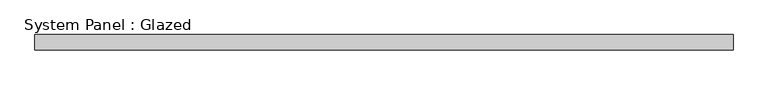
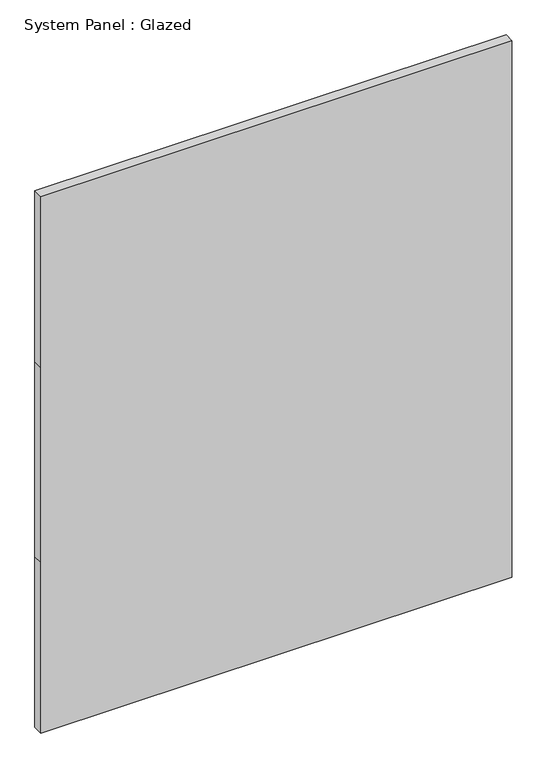
"""IFC4 building model written with IfcOpenShell, lengths in millimetres: plate geometry, System Panel : Glazed."""

from ifc_helpers import new_model, si_unit, frame, origin, place, context, project, spatial, polyline, outline, extrude, source, transform, mapped, element, save


def system_panel_glazed_93b0cd61(model_context):
    return source(origin(), model_context, "Body", "SweptSolid", [
        extrude(outline(polyline([(0.0, -587.375), (0.0, 587.375), (450.1068067, 587.375), (963.7136134, 587.375), (1413.8204201, 587.375), (1413.8204201, -587.375), (963.7136134, -587.375), (450.1068067, -587.375), (0.0, -587.375)])), frame((0.0, 19.05, 0.0), z_axis=(0.0, 1.0, 0.0), x_axis=(0.0, 0.0, 1.0)), (0.0, 0.0, 1.0), 25.4),
    ])


if __name__ == "__main__":
    model = new_model("IFC4")
    model_context = context("Model", 3, world=origin())
    ifc_project = project(units=[si_unit("LENGTHUNIT", "METRE", prefix="MILLI")], contexts=[model_context])
    site = spatial("IfcSite", under=ifc_project)
    building = spatial("IfcBuilding", under=site)
    placement = place(None, origin())
    system_panel_glazed_shape = system_panel_glazed_93b0cd61(model_context)
    element("IfcPlate", 1, ObjectType="System Panel : Glazed", at=placement, inside=building, context=model_context, shape_type="MappedRepresentation", body=[
        mapped(system_panel_glazed_shape, transform((0.0, 0.0, 0.0), x_axis=(1.0, 0.0, 0.0), y_axis=(0.0, 1.0, 0.0), z_axis=(0.0, 0.0, 1.0))),
    ])
    save(model, "model.ifc")

# Revit data of these elements
# Type "System Panel : Glazed"
#   Construction Type Id = "GSP4R"
#   Analytic Construction = "1/8 in Pilkington single glazing"
#   Visual Light Transmittance = 0.9
#   Solar Heat Gain Coefficient = 0.86
#   Heat Transfer Coefficient (U) = 1.18115 BTU/(h·ft²·°F)
#   Define Thermal Properties by = 1
# Element 1 (IfcPlate, "System Panel : Glazed")
#   Materials on its faces: "Glass"
# Materials
#   "Glass": class "Glass", colour RGB 0 128 192, transparency 0.75, Description = "Soda Lime Glass", Cost = 0
